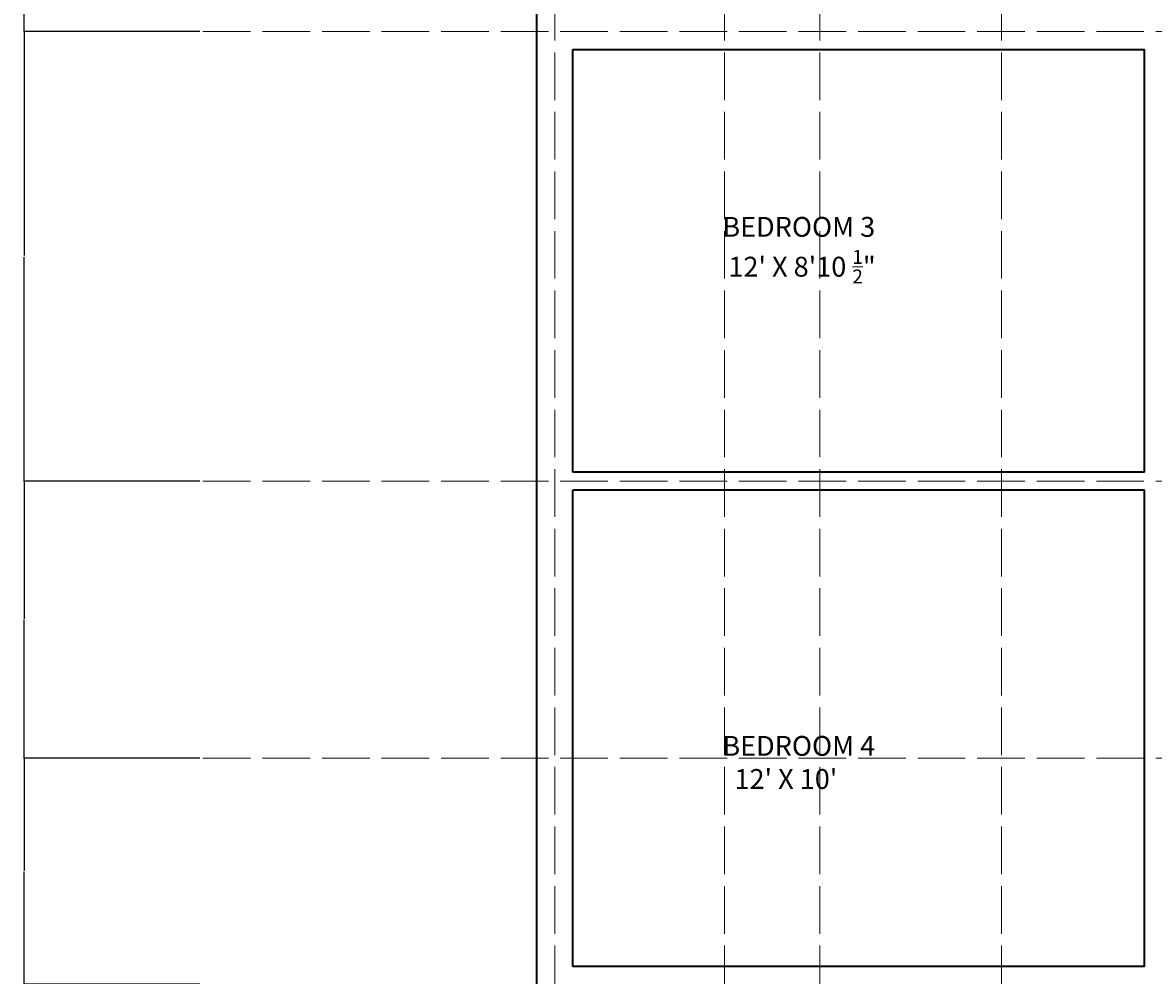
# Model space of a CAD drawing. Units: inches. Extents: x 1159 to 4240, y 1112 to 2085.
# Tile 2 of 13: x 1159 to 1443, y 1311 to 1551. Entities that reach past the tile are written whole.
import ezdxf

# ---------------------------------------------------------------- set-up
doc = ezdxf.new("R2010")
doc.units = ezdxf.units.IN
doc.linetypes.add('ACAD_ISO02W100', pattern=[15, 12, -3])
for name, color, linetype, lineweight in [('A-ANNO-DIMS', 2, 'Continuous', 18), ('A-AREA-IDEN', 30, 'Continuous', 18), ('A-GRID', 8, 'ACAD_ISO02W100', 13), ('WALL', 7, 'Continuous', 35)]:
    doc.layers.add(name, color=color, linetype=linetype, lineweight=lineweight)
doc.styles.get("Standard").update_dxf_attribs({"font": 'arial.ttf'})
doc.dimstyles.get("Standard").update_dxf_attribs({"dimtxt": 0.18, "dimasz": 0.18, "dimexe": 0.18, "dimexo": 0.0625, "dimgap": 0.09, "dimtad": 0, "dimtih": 1, "dimtoh": 1, "dimdec": 4, "dimzin": 0, "dimdsep": 46, "dimtxsty": 'Standard', "dimcen": 0.09, "dimadec": 0, "dimazin": 0, "dimtfac": 1, "dimtdec": 4, "dimtofl": 0, "dimtmove": 0, "dimatfit": 3, "dimfxl": 1, "dimtolj": 1, "dimtzin": 0, "dimarcsym": 0})

# ---------------------------------------------------------------- blocks, each defined once
blk = doc.blocks.new('HOUSE-35x60-WALL-LAYOUT')
for p, q in [((0, 0), (0, 720)), ((9, 297), (153, 297)), ((9, 190.5), (9, 297)), ((153, 190.5), (153, 297)), ((153, 190.5), (9, 190.5)), ((9, 66), (9, 186)), ((153, 186), (9, 186)), ((153, 66), (153, 186)), ((153, 66), (9, 66))]:
    blk.add_line(p, q)
blk = doc.blocks.new('HOUSE-35x60-SETTING-OUT-GRID')
for p, q in [((89.32, 0), (89.32, 883.25)), ((132.07, 0), (132.07, 883.25)), ((156.07, 0), (156.07, 883.25)), ((201.82, 0), (201.82, 883.25)), ((582.7, 392.25), (0, 392.25)), ((582.7, 279), (0, 279)), ((582.7, 209.25), (0, 209.25))]:
    blk.add_line(p, q)
blk = doc.blocks.new('*D38')
at = {"layer": 'A-ANNO-DIMS', "color": 0, "lineweight": -2, "transparency": 16777216}
for p, q in [((1203.25, 1366.2), (1158.78, 1366.2)), ((1158.96, 1366.02), (1158.96, 1337.88)), ((1158.96, 1309.38), (1158.96, 1337.52)), ((1203.25, 1309.2), (1158.78, 1309.2))]:
    blk.add_line(p, q, dxfattribs=at)
at = {"layer": 'A-ANNO-DIMS', "color": 0, "lineweight": 100, "transparency": 16777216}
for points in [[(1158.93, 1366.02), (1158.99, 1366.02), (1158.96, 1366.2)], [(1158.93, 1309.38), (1158.99, 1309.38), (1158.96, 1309.2)]]:
    blk.add_solid(points, dxfattribs=at)
at = {"layer": 'Defpoints', "color": 0, "lineweight": 100, "transparency": 16777216}
for p in [(1158.96, 1366.2), (1203.31, 1366.2), (1203.31, 1309.2)]:
    blk.add_point(p, dxfattribs=at)
at = {"layer": 'A-ANNO-DIMS', "color": 0, "transparency": 16777216, "insert": (1158.96, 1337.7), "char_height": 0.18, "attachment_point": 5}
blk.add_mtext('\\A1;57', dxfattribs=at)
blk = doc.blocks.new('*D39')
at = {"layer": 'A-ANNO-DIMS', "color": 0, "lineweight": -2, "transparency": 16777216}
for p, q in [((1203.25, 1435.95), (1158.78, 1435.95)), ((1158.96, 1435.77), (1158.96, 1401.26)), ((1158.96, 1366.38), (1158.96, 1400.9)), ((1203.25, 1366.2), (1158.78, 1366.2))]:
    blk.add_line(p, q, dxfattribs=at)
at = {"layer": 'A-ANNO-DIMS', "color": 0, "lineweight": 100, "transparency": 16777216}
for points in [[(1158.93, 1435.77), (1158.99, 1435.77), (1158.96, 1435.95)], [(1158.93, 1366.38), (1158.99, 1366.38), (1158.96, 1366.2)]]:
    blk.add_solid(points, dxfattribs=at)
at = {"layer": 'Defpoints', "color": 0, "lineweight": 100, "transparency": 16777216}
for p in [(1158.96, 1435.95), (1203.31, 1435.95), (1203.31, 1366.2)]:
    blk.add_point(p, dxfattribs=at)
at = {"layer": 'A-ANNO-DIMS', "color": 0, "transparency": 16777216, "insert": (1158.96, 1401.08), "char_height": 0.18, "attachment_point": 5}
blk.add_mtext('\\A1;69.75', dxfattribs=at)
blk = doc.blocks.new('*D40')
at = {"layer": 'A-ANNO-DIMS', "color": 0, "lineweight": -2, "transparency": 16777216}
for p, q in [((1203.25, 1549.2), (1158.78, 1549.2)), ((1158.96, 1549.02), (1158.96, 1492.76)), ((1158.96, 1436.13), (1158.96, 1492.4)), ((1203.25, 1435.95), (1158.78, 1435.95))]:
    blk.add_line(p, q, dxfattribs=at)
at = {"layer": 'A-ANNO-DIMS', "color": 0, "lineweight": 100, "transparency": 16777216}
for points in [[(1158.93, 1549.02), (1158.99, 1549.02), (1158.96, 1549.2)], [(1158.93, 1436.13), (1158.99, 1436.13), (1158.96, 1435.95)]]:
    blk.add_solid(points, dxfattribs=at)
at = {"layer": 'Defpoints', "color": 0, "lineweight": 100, "transparency": 16777216}
for p in [(1158.96, 1549.2), (1203.31, 1549.2), (1203.31, 1435.95)]:
    blk.add_point(p, dxfattribs=at)
at = {"layer": 'A-ANNO-DIMS', "color": 0, "transparency": 16777216, "insert": (1158.96, 1492.58), "char_height": 0.18, "attachment_point": 5}
blk.add_mtext('\\A1;113.25', dxfattribs=at)
blk = doc.blocks.new('*D41')
at = {"layer": 'A-ANNO-DIMS', "color": 0, "lineweight": -2, "transparency": 16777216}
for p, q in [((1203.25, 1671.45), (1158.78, 1671.45)), ((1158.96, 1671.27), (1158.96, 1610.51)), ((1158.96, 1549.38), (1158.96, 1610.15)), ((1203.25, 1549.2), (1158.78, 1549.2))]:
    blk.add_line(p, q, dxfattribs=at)
at = {"layer": 'A-ANNO-DIMS', "color": 0, "lineweight": 100, "transparency": 16777216}
for points in [[(1158.93, 1671.27), (1158.99, 1671.27), (1158.96, 1671.45)], [(1158.93, 1549.38), (1158.99, 1549.38), (1158.96, 1549.2)]]:
    blk.add_solid(points, dxfattribs=at)
at = {"layer": 'Defpoints', "color": 0, "lineweight": 100, "transparency": 16777216}
for p in [(1158.96, 1671.45), (1203.31, 1671.45), (1203.31, 1549.2)]:
    blk.add_point(p, dxfattribs=at)
at = {"layer": 'A-ANNO-DIMS', "color": 0, "transparency": 16777216, "insert": (1158.96, 1610.33), "char_height": 0.18, "attachment_point": 5}
blk.add_mtext('\\A1;122.25', dxfattribs=at)

msp = doc.modelspace()

# ---------------------------------------------------------------- block references
at = {"layer": 'A-GRID'}
msp.add_blockref('HOUSE-35x60-SETTING-OUT-GRID', (1203.31, 1156.954), dxfattribs=at)
at = {"layer": 'WALL'}
msp.add_blockref('HOUSE-35x60-WALL-LAYOUT', (1288.126, 1247.702), dxfattribs=at)

# ---------------------------------------------------------------- texts
at = {"layer": 'A-AREA-IDEN', "char_height": 5, "attachment_point": 1}
for s, insert in [('\\A1;BEDROOM 3\\P 12\' X 8\'10 {\\H0.7x;\\S1/2;}"', (1334.817, 1502.503)), ("\\A1;BEDROOM 4\\P  12' X 10'", (1334.817, 1371.76))]:
    msp.add_mtext_dynamic_manual_height_columns(s, width=140.18614, gutter_width=12.5, heights=[0], dxfattribs=dict(at, insert=insert))

# ---------------------------------------------------------------- dimensions: what is measured, and where the dimension line sits
at = {"layer": 'A-ANNO-DIMS'}
for base, p1, p2, override, picture, middle in [((1158.96, 1671.452), (1203.31, 1549.202), (1203.31, 1671.452), {"dimdec": 2, "dimlfac": 1, "dimrnd": 0, "dimzin": 0, "dimdsep": 46, "dimlunit": 2}, '*D41', (1158.96, 1610.327)), ((1158.96, 1549.202), (1203.31, 1435.952), (1203.31, 1549.202), {"dimdec": 2, "dimlfac": 1, "dimrnd": 0, "dimzin": 0, "dimdsep": 46, "dimlunit": 2}, '*D40', (1158.96, 1492.577)), ((1158.96, 1435.952), (1203.31, 1366.202), (1203.31, 1435.952), {"dimdec": 2, "dimlfac": 1, "dimrnd": 0, "dimzin": 0, "dimdsep": 46, "dimlunit": 2}, '*D39', (1158.96, 1401.077)), ((1158.96, 1366.202), (1203.31, 1309.202), (1203.31, 1366.202), {"dimdec": 0, "dimlfac": 1, "dimrnd": 0, "dimzin": 0, "dimdsep": 46, "dimlunit": 2}, '*D38', (1158.96, 1337.702))]:
    dim = msp.add_linear_dim(base=base, p1=p1, p2=p2, angle=90, dimstyle='Standard', override=override, dxfattribs=at)
    dim.commit()
    dim.dimension.update_dxf_attribs({"geometry": picture, "text_midpoint": middle})

doc.saveas('drawing.dxf')
